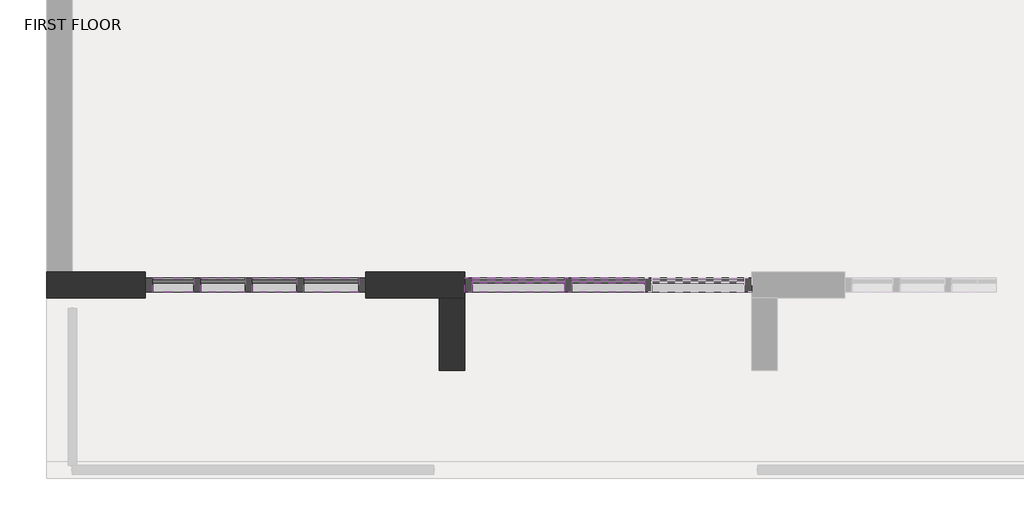
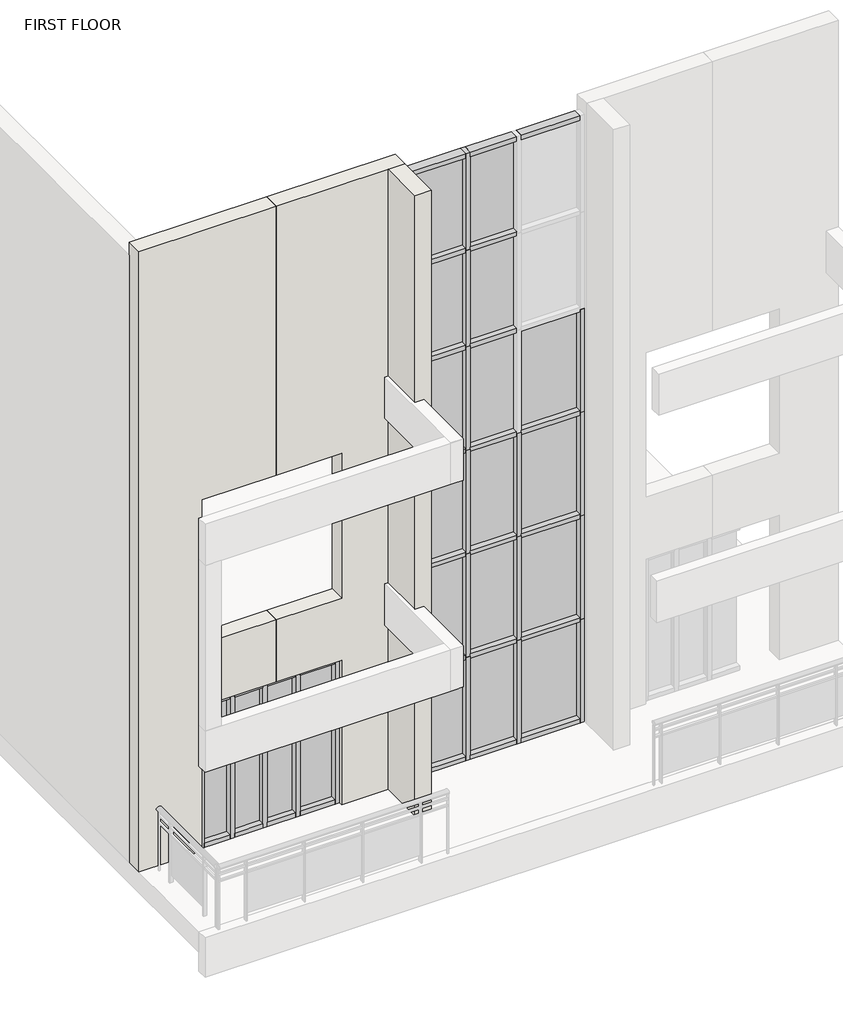
# One storey, part 1 of 2: 64 members, 24 plates, 3 walls.
"""IFC4 building model written with IfcOpenShell, lengths in millimetres."""

from ifc_helpers import new_model, si_unit, frame, origin, place, context, project, spatial, polyline, outline, extrude, faceted_brep, transform, mapped, element, save
from components import member_3374d9b6, member_c17f1be2, member_5215b92c, member_82905deb, member_ad567e07, member_e53b78c9, member_4491d118, member_0514ece2, member_5493b72c, member_7cbddb58, member_843225dc, member_7096a90e, member_499db0bc, system_panel_glazed_d26374ee, system_panel_glazed_59bf60dd, system_panel_glazed_016e6134, system_panel_glazed_b44f8fb5, system_panel_glazed_3f785c8f, system_panel_glazed_bf013b5c, system_panel_glazed_d91b2d6b, system_panel_glazed_ad4bb790, system_panel_glazed_935821d8, system_panel_glazed_f3f5655f, system_panel_glazed_1490133a

model = new_model("IFC4")

# Units and contexts
model_context = context("Model", 3, world=origin())
ifc_project = project(units=[si_unit("LENGTHUNIT", "METRE", prefix="MILLI")], contexts=[model_context])

# Site, building, storey
site = spatial("IfcSite", under=ifc_project)
building = spatial("IfcBuilding", under=site)
storey = spatial("IfcBuildingStorey", under=building, Name="FIRST FLOOR", Elevation=3048.0)

# Members
placement = place(None, origin())
member_shape = member_3374d9b6(model_context)
element("IfcMember", 1, ObjectType="Rectangular Mullion : 2.5\" x 5\" rectangular", at=placement, inside=storey, context=model_context, shape_type="MappedRepresentation", body=[
    mapped(member_shape, transform((-3493.058803, -508.3464931, 3048.0), x_axis=(1.0, 0.0, 0.0), y_axis=(0.0, -1.0, 0.0), z_axis=(0.0, 0.0, -1.0))),
])
element("IfcMember", 2, ObjectType="Rectangular Mullion : 2.5\" x 5\" rectangular", at=placement, inside=storey, context=model_context, shape_type="MappedRepresentation", body=[
    mapped(member_shape, transform((-3493.058803, -508.3464931, 3048.0), x_axis=(1.0, 0.0, 0.0), y_axis=(0.0, -1.0, 0.0), z_axis=(0.0, 0.0, -1.0))),
])
element("IfcMember", 3, ObjectType="Rectangular Mullion : 2.5\" x 5\" rectangular", at=placement, inside=storey, context=model_context, shape_type="MappedRepresentation", body=[
    mapped(member_shape, transform((-5445.7230786, -508.3464931, 5181.6), x_axis=(-1.0, 0.0, 0.0), y_axis=(0.0, -1.0, 0.0), z_axis=(0.0, 0.0, 1.0))),
])
element("IfcMember", 4, ObjectType="Rectangular Mullion : 2.5\" x 5\" rectangular", at=placement, inside=storey, context=model_context, shape_type="MappedRepresentation", body=[
    mapped(member_shape, transform((-5445.7230786, -508.3464931, 5181.6), x_axis=(-1.0, 0.0, 0.0), y_axis=(0.0, -1.0, 0.0), z_axis=(0.0, 0.0, 1.0))),
])
member_2_shape = member_c17f1be2(model_context)
element("IfcMember", 5, ObjectType="Rectangular Mullion : 2.5\" x 5\" rectangular", at=placement, inside=storey, context=model_context, shape_type="MappedRepresentation", body=[
    mapped(member_2_shape, transform((-2553.258803, -508.3464931, 3048.0), x_axis=(0.0, 0.0, -1.0), y_axis=(0.0, -1.0, 0.0), z_axis=(-1.0, 0.0, 0.0))),
])
element("IfcMember", 6, ObjectType="Rectangular Mullion : 2.5\" x 5\" rectangular", at=placement, inside=storey, context=model_context, shape_type="MappedRepresentation", body=[
    mapped(member_2_shape, transform((-959.408803, -508.3464931, 3048.0), x_axis=(0.0, 0.0, -1.0), y_axis=(0.0, -1.0, 0.0), z_axis=(-1.0, 0.0, 0.0))),
])
element("IfcMember", 7, ObjectType="Rectangular Mullion : 2.5\" x 5\" rectangular", at=placement, inside=storey, context=model_context, shape_type="MappedRepresentation", body=[
    mapped(member_2_shape, transform((-140.258803, -508.3464931, 12000.3983116), x_axis=(0.0, 0.0, 1.0), y_axis=(0.0, -1.0, 0.0), z_axis=(1.0, 0.0, 0.0))),
])
element("IfcMember", 8, ObjectType="Rectangular Mullion : 2.5\" x 5\" rectangular", at=placement, inside=storey, context=model_context, shape_type="MappedRepresentation", body=[
    mapped(member_2_shape, transform((-1734.108803, -508.3464931, 12000.3983116), x_axis=(0.0, 0.0, 1.0), y_axis=(0.0, -1.0, 0.0), z_axis=(1.0, 0.0, 0.0))),
])
member_3_shape = member_5215b92c(model_context)
element("IfcMember", 9, ObjectType="Rectangular Mullion : 2.5\" x 5\" rectangular", at=placement, inside=storey, context=model_context, shape_type="MappedRepresentation", body=[
    mapped(member_3_shape, transform((-1670.608803, -508.3464931, 3048.0), x_axis=(0.0, 0.0, -1.0), y_axis=(0.0, -1.0, 0.0), z_axis=(-1.0, 0.0, 0.0))),
])
element("IfcMember", 10, ObjectType="Rectangular Mullion : 2.5\" x 5\" rectangular", at=placement, inside=storey, context=model_context, shape_type="MappedRepresentation", body=[
    mapped(member_3_shape, transform((-1022.908803, -508.3464931, 12000.3983116), x_axis=(0.0, 0.0, 1.0), y_axis=(0.0, -1.0, 0.0), z_axis=(1.0, 0.0, 0.0))),
])
member_4_shape = member_82905deb(model_context)
element("IfcMember", 11, ObjectType="Rectangular Mullion : 2.5\" x 5\" rectangular", at=placement, inside=storey, context=model_context, shape_type="MappedRepresentation", body=[
    mapped(member_4_shape, transform((-1702.358803, -508.3464931, 3048.0), x_axis=(1.0, 0.0, 0.0), y_axis=(0.0, -1.0, 0.0), z_axis=(0.0, 0.0, -1.0))),
])
element("IfcMember", 12, ObjectType="Rectangular Mullion : 2.5\" x 5\" rectangular", at=placement, inside=storey, context=model_context, shape_type="MappedRepresentation", body=[
    mapped(member_4_shape, transform((-991.158803, -508.3464931, 3048.0), x_axis=(1.0, 0.0, 0.0), y_axis=(0.0, -1.0, 0.0), z_axis=(0.0, 0.0, -1.0))),
])
member_5_shape = member_ad567e07(model_context)
element("IfcMember", 13, ObjectType="Rectangular Mullion : 2.5\" x 5\" rectangular", at=placement, inside=storey, context=model_context, shape_type="MappedRepresentation", body=[
    mapped(member_5_shape, transform((-1734.108803, -508.3464931, 4572.0), x_axis=(0.0, 0.0, 1.0), y_axis=(0.0, -1.0, 0.0), z_axis=(1.0, 0.0, 0.0))),
])
element("IfcMember", 14, ObjectType="Rectangular Mullion : 2.5\" x 5\" rectangular", at=placement, inside=storey, context=model_context, shape_type="MappedRepresentation", body=[
    mapped(member_5_shape, transform((-140.258803, -508.3464931, 4572.0), x_axis=(0.0, 0.0, 1.0), y_axis=(0.0, -1.0, 0.0), z_axis=(1.0, 0.0, 0.0))),
])
element("IfcMember", 15, ObjectType="Rectangular Mullion : 2.5\" x 5\" rectangular", at=placement, inside=storey, context=model_context, shape_type="MappedRepresentation", body=[
    mapped(member_5_shape, transform((-1734.108803, -508.3464931, 6096.0), x_axis=(0.0, 0.0, 1.0), y_axis=(0.0, -1.0, 0.0), z_axis=(1.0, 0.0, 0.0))),
])
element("IfcMember", 16, ObjectType="Rectangular Mullion : 2.5\" x 5\" rectangular", at=placement, inside=storey, context=model_context, shape_type="MappedRepresentation", body=[
    mapped(member_5_shape, transform((-140.258803, -508.3464931, 6096.0), x_axis=(0.0, 0.0, 1.0), y_axis=(0.0, -1.0, 0.0), z_axis=(1.0, 0.0, 0.0))),
])
element("IfcMember", 17, ObjectType="Rectangular Mullion : 2.5\" x 5\" rectangular", at=placement, inside=storey, context=model_context, shape_type="MappedRepresentation", body=[
    mapped(member_5_shape, transform((-1734.108803, -508.3464931, 7620.0), x_axis=(0.0, 0.0, 1.0), y_axis=(0.0, -1.0, 0.0), z_axis=(1.0, 0.0, 0.0))),
])
element("IfcMember", 18, ObjectType="Rectangular Mullion : 2.5\" x 5\" rectangular", at=placement, inside=storey, context=model_context, shape_type="MappedRepresentation", body=[
    mapped(member_5_shape, transform((-140.258803, -508.3464931, 7620.0), x_axis=(0.0, 0.0, 1.0), y_axis=(0.0, -1.0, 0.0), z_axis=(1.0, 0.0, 0.0))),
])
element("IfcMember", 19, ObjectType="Rectangular Mullion : 2.5\" x 5\" rectangular", at=placement, inside=storey, context=model_context, shape_type="MappedRepresentation", body=[
    mapped(member_5_shape, transform((-1734.108803, -508.3464931, 9144.0), x_axis=(0.0, 0.0, 1.0), y_axis=(0.0, -1.0, 0.0), z_axis=(1.0, 0.0, 0.0))),
])
element("IfcMember", 20, ObjectType="Rectangular Mullion : 2.5\" x 5\" rectangular", at=placement, inside=storey, context=model_context, shape_type="MappedRepresentation", body=[
    mapped(member_5_shape, transform((-1734.108803, -508.3464931, 10572.1991558), x_axis=(0.0, 0.0, 1.0), y_axis=(0.0, -1.0, 0.0), z_axis=(1.0, 0.0, 0.0))),
])
member_6_shape = member_e53b78c9(model_context)
element("IfcMember", 21, ObjectType="Rectangular Mullion : 2.5\" x 5\" rectangular", at=placement, inside=storey, context=model_context, shape_type="MappedRepresentation", body=[
    mapped(member_6_shape, transform((-1022.908803, -508.3464931, 4572.0), x_axis=(0.0, 0.0, 1.0), y_axis=(0.0, -1.0, 0.0), z_axis=(1.0, 0.0, 0.0))),
])
element("IfcMember", 22, ObjectType="Rectangular Mullion : 2.5\" x 5\" rectangular", at=placement, inside=storey, context=model_context, shape_type="MappedRepresentation", body=[
    mapped(member_6_shape, transform((-1022.908803, -508.3464931, 6096.0), x_axis=(0.0, 0.0, 1.0), y_axis=(0.0, -1.0, 0.0), z_axis=(1.0, 0.0, 0.0))),
])
element("IfcMember", 23, ObjectType="Rectangular Mullion : 2.5\" x 5\" rectangular", at=placement, inside=storey, context=model_context, shape_type="MappedRepresentation", body=[
    mapped(member_6_shape, transform((-1022.908803, -508.3464931, 7620.0), x_axis=(0.0, 0.0, 1.0), y_axis=(0.0, -1.0, 0.0), z_axis=(1.0, 0.0, 0.0))),
])
element("IfcMember", 24, ObjectType="Rectangular Mullion : 2.5\" x 5\" rectangular", at=placement, inside=storey, context=model_context, shape_type="MappedRepresentation", body=[
    mapped(member_6_shape, transform((-1022.908803, -508.3464931, 9144.0), x_axis=(0.0, 0.0, 1.0), y_axis=(0.0, -1.0, 0.0), z_axis=(1.0, 0.0, 0.0))),
])
element("IfcMember", 25, ObjectType="Rectangular Mullion : 2.5\" x 5\" rectangular", at=placement, inside=storey, context=model_context, shape_type="MappedRepresentation", body=[
    mapped(member_6_shape, transform((-1022.908803, -508.3464931, 10572.1991558), x_axis=(0.0, 0.0, 1.0), y_axis=(0.0, -1.0, 0.0), z_axis=(1.0, 0.0, 0.0))),
])
member_7_shape = member_4491d118(model_context)
element("IfcMember", 26, ObjectType="Rectangular Mullion : 2.5\" x 5\" rectangular", at=placement, inside=storey, context=model_context, shape_type="MappedRepresentation", body=[
    mapped(member_7_shape, transform((-76.758803, -508.3464931, 3048.0), x_axis=(1.0, 0.0, 0.0), y_axis=(0.0, -1.0, 0.0), z_axis=(0.0, 0.0, -1.0))),
])
element("IfcMember", 27, ObjectType="Rectangular Mullion : 2.5\" x 5\" rectangular", at=placement, inside=storey, context=model_context, shape_type="MappedRepresentation", body=[
    mapped(member_7_shape, transform((-2616.758803, -508.3464931, 4572.0), x_axis=(-1.0, 0.0, 0.0), y_axis=(0.0, -1.0, 0.0), z_axis=(0.0, 0.0, 1.0))),
])
element("IfcMember", 28, ObjectType="Rectangular Mullion : 2.5\" x 5\" rectangular", at=placement, inside=storey, context=model_context, shape_type="MappedRepresentation", body=[
    mapped(member_4_shape, transform((-1702.358803, -508.3464931, 4572.0), x_axis=(1.0, 0.0, 0.0), y_axis=(0.0, -1.0, 0.0), z_axis=(0.0, 0.0, -1.0))),
])
element("IfcMember", 29, ObjectType="Rectangular Mullion : 2.5\" x 5\" rectangular", at=placement, inside=storey, context=model_context, shape_type="MappedRepresentation", body=[
    mapped(member_4_shape, transform((-991.158803, -508.3464931, 4572.0), x_axis=(1.0, 0.0, 0.0), y_axis=(0.0, -1.0, 0.0), z_axis=(0.0, 0.0, -1.0))),
])
element("IfcMember", 30, ObjectType="Rectangular Mullion : 2.5\" x 5\" rectangular", at=placement, inside=storey, context=model_context, shape_type="MappedRepresentation", body=[
    mapped(member_4_shape, transform((-1702.358803, -508.3464931, 6096.0), x_axis=(1.0, 0.0, 0.0), y_axis=(0.0, -1.0, 0.0), z_axis=(0.0, 0.0, -1.0))),
])
element("IfcMember", 31, ObjectType="Rectangular Mullion : 2.5\" x 5\" rectangular", at=placement, inside=storey, context=model_context, shape_type="MappedRepresentation", body=[
    mapped(member_4_shape, transform((-991.158803, -508.3464931, 6096.0), x_axis=(1.0, 0.0, 0.0), y_axis=(0.0, -1.0, 0.0), z_axis=(0.0, 0.0, -1.0))),
])
element("IfcMember", 32, ObjectType="Rectangular Mullion : 2.5\" x 5\" rectangular", at=placement, inside=storey, context=model_context, shape_type="MappedRepresentation", body=[
    mapped(member_4_shape, transform((-1702.358803, -508.3464931, 7620.0), x_axis=(1.0, 0.0, 0.0), y_axis=(0.0, -1.0, 0.0), z_axis=(0.0, 0.0, -1.0))),
])
element("IfcMember", 33, ObjectType="Rectangular Mullion : 2.5\" x 5\" rectangular", at=placement, inside=storey, context=model_context, shape_type="MappedRepresentation", body=[
    mapped(member_7_shape, transform((-76.758803, -508.3464931, 4572.0), x_axis=(1.0, 0.0, 0.0), y_axis=(0.0, -1.0, 0.0), z_axis=(0.0, 0.0, -1.0))),
])
element("IfcMember", 34, ObjectType="Rectangular Mullion : 2.5\" x 5\" rectangular", at=placement, inside=storey, context=model_context, shape_type="MappedRepresentation", body=[
    mapped(member_7_shape, transform((-76.758803, -508.3464931, 6096.0), x_axis=(1.0, 0.0, 0.0), y_axis=(0.0, -1.0, 0.0), z_axis=(0.0, 0.0, -1.0))),
])
element("IfcMember", 35, ObjectType="Rectangular Mullion : 2.5\" x 5\" rectangular", at=placement, inside=storey, context=model_context, shape_type="MappedRepresentation", body=[
    mapped(member_7_shape, transform((-76.758803, -508.3464931, 7620.0), x_axis=(1.0, 0.0, 0.0), y_axis=(0.0, -1.0, 0.0), z_axis=(0.0, 0.0, -1.0))),
])
element("IfcMember", 36, ObjectType="Rectangular Mullion : 2.5\" x 5\" rectangular", at=placement, inside=storey, context=model_context, shape_type="MappedRepresentation", body=[
    mapped(member_7_shape, transform((-2616.758803, -508.3464931, 6096.0), x_axis=(-1.0, 0.0, 0.0), y_axis=(0.0, -1.0, 0.0), z_axis=(0.0, 0.0, 1.0))),
])
element("IfcMember", 37, ObjectType="Rectangular Mullion : 2.5\" x 5\" rectangular", at=placement, inside=storey, context=model_context, shape_type="MappedRepresentation", body=[
    mapped(member_7_shape, transform((-2616.758803, -508.3464931, 7620.0), x_axis=(-1.0, 0.0, 0.0), y_axis=(0.0, -1.0, 0.0), z_axis=(0.0, 0.0, 1.0))),
])
element("IfcMember", 38, ObjectType="Rectangular Mullion : 2.5\" x 5\" rectangular", at=placement, inside=storey, context=model_context, shape_type="MappedRepresentation", body=[
    mapped(member_7_shape, transform((-2616.758803, -508.3464931, 9144.0), x_axis=(-1.0, 0.0, 0.0), y_axis=(0.0, -1.0, 0.0), z_axis=(0.0, 0.0, 1.0))),
])
member_8_shape = member_0514ece2(model_context)
element("IfcMember", 39, ObjectType="Rectangular Mullion : 2.5\" x 5\" rectangular", at=placement, inside=storey, context=model_context, shape_type="MappedRepresentation", body=[
    mapped(member_8_shape, transform((-1702.358803, -508.3464931, 9144.0), x_axis=(1.0, 0.0, 0.0), y_axis=(0.0, -1.0, 0.0), z_axis=(0.0, 0.0, -1.0))),
])
element("IfcMember", 40, ObjectType="Rectangular Mullion : 2.5\" x 5\" rectangular", at=placement, inside=storey, context=model_context, shape_type="MappedRepresentation", body=[
    mapped(member_8_shape, transform((-1702.358803, -508.3464931, 10572.1991558), x_axis=(1.0, 0.0, 0.0), y_axis=(0.0, -1.0, 0.0), z_axis=(0.0, 0.0, -1.0))),
])
member_9_shape = member_5493b72c(model_context)
element("IfcMember", 41, ObjectType="Rectangular Mullion : 2.5\" x 5\" rectangular", at=placement, inside=storey, context=model_context, shape_type="MappedRepresentation", body=[
    mapped(member_9_shape, transform((-2616.758803, -508.3464931, 12000.3983116), x_axis=(-1.0, 0.0, 0.0), y_axis=(0.0, -1.0, 0.0), z_axis=(0.0, 0.0, 1.0))),
])
element("IfcMember", 42, ObjectType="Rectangular Mullion : 2.5\" x 5\" rectangular", at=placement, inside=storey, context=model_context, shape_type="MappedRepresentation", body=[
    mapped(member_9_shape, transform((-2616.758803, -508.3464931, 10572.1991558), x_axis=(-1.0, 0.0, 0.0), y_axis=(0.0, -1.0, 0.0), z_axis=(0.0, 0.0, 1.0))),
])
member_10_shape = member_7cbddb58(model_context)
element("IfcMember", 43, ObjectType="Rectangular Mullion : 2.5\" x 5\" rectangular", at=placement, inside=storey, context=model_context, shape_type="MappedRepresentation", body=[
    mapped(member_10_shape, transform((-4988.5230786, -508.3464931, 3048.0), x_axis=(1.0, 0.0, 0.0), y_axis=(0.0, -1.0, 0.0), z_axis=(0.0, 0.0, -1.0))),
])
element("IfcMember", 44, ObjectType="Rectangular Mullion : 2.5\" x 5\" rectangular", at=placement, inside=storey, context=model_context, shape_type="MappedRepresentation", body=[
    mapped(member_10_shape, transform((-4531.3230786, -508.3464931, 3048.0), x_axis=(1.0, 0.0, 0.0), y_axis=(0.0, -1.0, 0.0), z_axis=(0.0, 0.0, -1.0))),
])
element("IfcMember", 45, ObjectType="Rectangular Mullion : 2.5\" x 5\" rectangular", at=placement, inside=storey, context=model_context, shape_type="MappedRepresentation", body=[
    mapped(member_10_shape, transform((-4074.1230786, -508.3464931, 3048.0), x_axis=(1.0, 0.0, 0.0), y_axis=(0.0, -1.0, 0.0), z_axis=(0.0, 0.0, -1.0))),
])
element("IfcMember", 46, ObjectType="Rectangular Mullion : 2.5\" x 5\" rectangular", at=placement, inside=storey, context=model_context, shape_type="MappedRepresentation", body=[
    mapped(member_10_shape, transform((-4988.5230786, -508.3464931, 3048.0), x_axis=(1.0, 0.0, 0.0), y_axis=(0.0, -1.0, 0.0), z_axis=(0.0, 0.0, -1.0))),
])
element("IfcMember", 47, ObjectType="Rectangular Mullion : 2.5\" x 5\" rectangular", at=placement, inside=storey, context=model_context, shape_type="MappedRepresentation", body=[
    mapped(member_10_shape, transform((-4531.3230786, -508.3464931, 3048.0), x_axis=(1.0, 0.0, 0.0), y_axis=(0.0, -1.0, 0.0), z_axis=(0.0, 0.0, -1.0))),
])
element("IfcMember", 48, ObjectType="Rectangular Mullion : 2.5\" x 5\" rectangular", at=placement, inside=storey, context=model_context, shape_type="MappedRepresentation", body=[
    mapped(member_10_shape, transform((-4074.1230786, -508.3464931, 3048.0), x_axis=(1.0, 0.0, 0.0), y_axis=(0.0, -1.0, 0.0), z_axis=(0.0, 0.0, -1.0))),
])
member_11_shape = member_843225dc(model_context)
element("IfcMember", 49, ObjectType="Rectangular Mullion : 2.5\" x 5\" rectangular", at=placement, inside=storey, context=model_context, shape_type="MappedRepresentation", body=[
    mapped(member_11_shape, transform((-5382.2230786, -508.3464931, 3048.0), x_axis=(0.0, 0.0, -1.0), y_axis=(0.0, -1.0, 0.0), z_axis=(-1.0, 0.0, 0.0))),
])
element("IfcMember", 50, ObjectType="Rectangular Mullion : 2.5\" x 5\" rectangular", at=placement, inside=storey, context=model_context, shape_type="MappedRepresentation", body=[
    mapped(member_11_shape, transform((-5382.2230786, -508.3464931, 3048.0), x_axis=(0.0, 0.0, -1.0), y_axis=(0.0, -1.0, 0.0), z_axis=(-1.0, 0.0, 0.0))),
])
element("IfcMember", 51, ObjectType="Rectangular Mullion : 2.5\" x 5\" rectangular", at=placement, inside=storey, context=model_context, shape_type="MappedRepresentation", body=[
    mapped(member_11_shape, transform((-5020.2730786, -508.3464931, 5181.6), x_axis=(0.0, 0.0, 1.0), y_axis=(0.0, -1.0, 0.0), z_axis=(1.0, 0.0, 0.0))),
])
element("IfcMember", 52, ObjectType="Rectangular Mullion : 2.5\" x 5\" rectangular", at=placement, inside=storey, context=model_context, shape_type="MappedRepresentation", body=[
    mapped(member_11_shape, transform((-5020.2730786, -508.3464931, 5181.6), x_axis=(0.0, 0.0, 1.0), y_axis=(0.0, -1.0, 0.0), z_axis=(1.0, 0.0, 0.0))),
])
member_12_shape = member_7096a90e(model_context)
element("IfcMember", 53, ObjectType="Rectangular Mullion : 2.5\" x 5\" rectangular", at=placement, inside=storey, context=model_context, shape_type="MappedRepresentation", body=[
    mapped(member_12_shape, transform((-4956.7730786, -508.3464931, 3048.0), x_axis=(0.0, 0.0, -1.0), y_axis=(0.0, -1.0, 0.0), z_axis=(-1.0, 0.0, 0.0))),
])
element("IfcMember", 54, ObjectType="Rectangular Mullion : 2.5\" x 5\" rectangular", at=placement, inside=storey, context=model_context, shape_type="MappedRepresentation", body=[
    mapped(member_12_shape, transform((-4499.5730786, -508.3464931, 3048.0), x_axis=(0.0, 0.0, -1.0), y_axis=(0.0, -1.0, 0.0), z_axis=(-1.0, 0.0, 0.0))),
])
element("IfcMember", 55, ObjectType="Rectangular Mullion : 2.5\" x 5\" rectangular", at=placement, inside=storey, context=model_context, shape_type="MappedRepresentation", body=[
    mapped(member_12_shape, transform((-4956.7730786, -508.3464931, 3048.0), x_axis=(0.0, 0.0, -1.0), y_axis=(0.0, -1.0, 0.0), z_axis=(-1.0, 0.0, 0.0))),
])
element("IfcMember", 56, ObjectType="Rectangular Mullion : 2.5\" x 5\" rectangular", at=placement, inside=storey, context=model_context, shape_type="MappedRepresentation", body=[
    mapped(member_12_shape, transform((-4499.5730786, -508.3464931, 3048.0), x_axis=(0.0, 0.0, -1.0), y_axis=(0.0, -1.0, 0.0), z_axis=(-1.0, 0.0, 0.0))),
])
element("IfcMember", 57, ObjectType="Rectangular Mullion : 2.5\" x 5\" rectangular", at=placement, inside=storey, context=model_context, shape_type="MappedRepresentation", body=[
    mapped(member_12_shape, transform((-4563.0730786, -508.3464931, 5181.6), x_axis=(0.0, 0.0, 1.0), y_axis=(0.0, -1.0, 0.0), z_axis=(1.0, 0.0, 0.0))),
])
element("IfcMember", 58, ObjectType="Rectangular Mullion : 2.5\" x 5\" rectangular", at=placement, inside=storey, context=model_context, shape_type="MappedRepresentation", body=[
    mapped(member_12_shape, transform((-4105.8730786, -508.3464931, 5181.6), x_axis=(0.0, 0.0, 1.0), y_axis=(0.0, -1.0, 0.0), z_axis=(1.0, 0.0, 0.0))),
])
element("IfcMember", 59, ObjectType="Rectangular Mullion : 2.5\" x 5\" rectangular", at=placement, inside=storey, context=model_context, shape_type="MappedRepresentation", body=[
    mapped(member_12_shape, transform((-4563.0730786, -508.3464931, 5181.6), x_axis=(0.0, 0.0, 1.0), y_axis=(0.0, -1.0, 0.0), z_axis=(1.0, 0.0, 0.0))),
])
element("IfcMember", 60, ObjectType="Rectangular Mullion : 2.5\" x 5\" rectangular", at=placement, inside=storey, context=model_context, shape_type="MappedRepresentation", body=[
    mapped(member_12_shape, transform((-4105.8730786, -508.3464931, 5181.6), x_axis=(0.0, 0.0, 1.0), y_axis=(0.0, -1.0, 0.0), z_axis=(1.0, 0.0, 0.0))),
])
member_13_shape = member_499db0bc(model_context)
element("IfcMember", 61, ObjectType="Rectangular Mullion : 2.5\" x 5\" rectangular", at=placement, inside=storey, context=model_context, shape_type="MappedRepresentation", body=[
    mapped(member_13_shape, transform((-3556.558803, -508.3464931, 5181.6), x_axis=(0.0, 0.0, 1.0), y_axis=(0.0, -1.0, 0.0), z_axis=(1.0, 0.0, 0.0))),
])
element("IfcMember", 62, ObjectType="Rectangular Mullion : 2.5\" x 5\" rectangular", at=placement, inside=storey, context=model_context, shape_type="MappedRepresentation", body=[
    mapped(member_13_shape, transform((-3556.558803, -508.3464931, 5181.6), x_axis=(0.0, 0.0, 1.0), y_axis=(0.0, -1.0, 0.0), z_axis=(1.0, 0.0, 0.0))),
])
element("IfcMember", 63, ObjectType="Rectangular Mullion : 2.5\" x 5\" rectangular", at=placement, inside=storey, context=model_context, shape_type="MappedRepresentation", body=[
    mapped(member_13_shape, transform((-4042.3730786, -508.3464931, 3048.0), x_axis=(0.0, 0.0, -1.0), y_axis=(0.0, -1.0, 0.0), z_axis=(-1.0, 0.0, 0.0))),
])
element("IfcMember", 64, ObjectType="Rectangular Mullion : 2.5\" x 5\" rectangular", at=placement, inside=storey, context=model_context, shape_type="MappedRepresentation", body=[
    mapped(member_13_shape, transform((-4042.3730786, -508.3464931, 3048.0), x_axis=(0.0, 0.0, -1.0), y_axis=(0.0, -1.0, 0.0), z_axis=(-1.0, 0.0, 0.0))),
])

# Plates
system_panel_glazed_shape = system_panel_glazed_d26374ee(model_context)
element("IfcPlate", 65, ObjectType="System Panel : Glazed", at=placement, inside=storey, context=model_context, shape_type="MappedRepresentation", body=[
    mapped(system_panel_glazed_shape, transform((-2143.683803, -508.3464931, 3111.5), x_axis=(1.0, 0.0, 0.0), y_axis=(0.0, 1.0, 0.0), z_axis=(0.0, 0.0, 1.0))),
])
element("IfcPlate", 66, ObjectType="System Panel : Glazed", at=placement, inside=storey, context=model_context, shape_type="MappedRepresentation", body=[
    mapped(system_panel_glazed_shape, transform((-549.833803, -508.3464931, 3111.5), x_axis=(1.0, 0.0, 0.0), y_axis=(0.0, 1.0, 0.0), z_axis=(0.0, 0.0, 1.0))),
])
system_panel_glazed_2_shape = system_panel_glazed_59bf60dd(model_context)
element("IfcPlate", 67, ObjectType="System Panel : Glazed", at=placement, inside=storey, context=model_context, shape_type="MappedRepresentation", body=[
    mapped(system_panel_glazed_2_shape, transform((-1346.758803, -508.3464931, 3111.5), x_axis=(1.0, 0.0, 0.0), y_axis=(0.0, 1.0, 0.0), z_axis=(0.0, 0.0, 1.0))),
])
system_panel_glazed_3_shape = system_panel_glazed_016e6134(model_context)
element("IfcPlate", 68, ObjectType="System Panel : Glazed", at=placement, inside=storey, context=model_context, shape_type="MappedRepresentation", body=[
    mapped(system_panel_glazed_3_shape, transform((-2143.683803, -508.3464931, 4603.75), x_axis=(1.0, 0.0, 0.0), y_axis=(0.0, 1.0, 0.0), z_axis=(0.0, 0.0, 1.0))),
])
element("IfcPlate", 69, ObjectType="System Panel : Glazed", at=placement, inside=storey, context=model_context, shape_type="MappedRepresentation", body=[
    mapped(system_panel_glazed_3_shape, transform((-549.833803, -508.3464931, 4603.75), x_axis=(1.0, 0.0, 0.0), y_axis=(0.0, 1.0, 0.0), z_axis=(0.0, 0.0, 1.0))),
])
element("IfcPlate", 70, ObjectType="System Panel : Glazed", at=placement, inside=storey, context=model_context, shape_type="MappedRepresentation", body=[
    mapped(system_panel_glazed_3_shape, transform((-2143.683803, -508.3464931, 6127.75), x_axis=(1.0, 0.0, 0.0), y_axis=(0.0, 1.0, 0.0), z_axis=(0.0, 0.0, 1.0))),
])
element("IfcPlate", 71, ObjectType="System Panel : Glazed", at=placement, inside=storey, context=model_context, shape_type="MappedRepresentation", body=[
    mapped(system_panel_glazed_3_shape, transform((-549.833803, -508.3464931, 6127.75), x_axis=(1.0, 0.0, 0.0), y_axis=(0.0, 1.0, 0.0), z_axis=(0.0, 0.0, 1.0))),
])
element("IfcPlate", 72, ObjectType="System Panel : Glazed", at=placement, inside=storey, context=model_context, shape_type="MappedRepresentation", body=[
    mapped(system_panel_glazed_3_shape, transform((-2143.683803, -508.3464931, 7651.75), x_axis=(1.0, 0.0, 0.0), y_axis=(0.0, 1.0, 0.0), z_axis=(0.0, 0.0, 1.0))),
])
element("IfcPlate", 73, ObjectType="System Panel : Glazed", at=placement, inside=storey, context=model_context, shape_type="MappedRepresentation", body=[
    mapped(system_panel_glazed_3_shape, transform((-549.833803, -508.3464931, 7651.75), x_axis=(1.0, 0.0, 0.0), y_axis=(0.0, 1.0, 0.0), z_axis=(0.0, 0.0, 1.0))),
])
system_panel_glazed_4_shape = system_panel_glazed_b44f8fb5(model_context)
element("IfcPlate", 74, ObjectType="System Panel : Glazed", at=placement, inside=storey, context=model_context, shape_type="MappedRepresentation", body=[
    mapped(system_panel_glazed_4_shape, transform((-1346.758803, -508.3464931, 4603.75), x_axis=(1.0, 0.0, 0.0), y_axis=(0.0, 1.0, 0.0), z_axis=(0.0, 0.0, 1.0))),
])
element("IfcPlate", 75, ObjectType="System Panel : Glazed", at=placement, inside=storey, context=model_context, shape_type="MappedRepresentation", body=[
    mapped(system_panel_glazed_4_shape, transform((-1346.758803, -508.3464931, 6127.75), x_axis=(1.0, 0.0, 0.0), y_axis=(0.0, 1.0, 0.0), z_axis=(0.0, 0.0, 1.0))),
])
element("IfcPlate", 76, ObjectType="System Panel : Glazed", at=placement, inside=storey, context=model_context, shape_type="MappedRepresentation", body=[
    mapped(system_panel_glazed_4_shape, transform((-1346.758803, -508.3464931, 7651.75), x_axis=(1.0, 0.0, 0.0), y_axis=(0.0, 1.0, 0.0), z_axis=(0.0, 0.0, 1.0))),
])
system_panel_glazed_5_shape = system_panel_glazed_3f785c8f(model_context)
element("IfcPlate", 77, ObjectType="System Panel : Glazed", at=placement, inside=storey, context=model_context, shape_type="MappedRepresentation", body=[
    mapped(system_panel_glazed_5_shape, transform((-2143.683803, -508.3464931, 9175.75), x_axis=(1.0, 0.0, 0.0), y_axis=(0.0, 1.0, 0.0), z_axis=(0.0, 0.0, 1.0))),
])
system_panel_glazed_6_shape = system_panel_glazed_bf013b5c(model_context)
element("IfcPlate", 78, ObjectType="System Panel : Glazed", at=placement, inside=storey, context=model_context, shape_type="MappedRepresentation", body=[
    mapped(system_panel_glazed_6_shape, transform((-1346.758803, -508.3464931, 9175.75), x_axis=(1.0, 0.0, 0.0), y_axis=(0.0, 1.0, 0.0), z_axis=(0.0, 0.0, 1.0))),
])
system_panel_glazed_7_shape = system_panel_glazed_d91b2d6b(model_context)
element("IfcPlate", 79, ObjectType="System Panel : Glazed", at=placement, inside=storey, context=model_context, shape_type="MappedRepresentation", body=[
    mapped(system_panel_glazed_7_shape, transform((-2143.683803, -508.3464931, 10603.9491558), x_axis=(1.0, 0.0, 0.0), y_axis=(0.0, 1.0, 0.0), z_axis=(0.0, 0.0, 1.0))),
])
system_panel_glazed_8_shape = system_panel_glazed_ad4bb790(model_context)
element("IfcPlate", 80, ObjectType="System Panel : Glazed", at=placement, inside=storey, context=model_context, shape_type="MappedRepresentation", body=[
    mapped(system_panel_glazed_8_shape, transform((-1346.758803, -508.3464931, 10603.9491558), x_axis=(1.0, 0.0, 0.0), y_axis=(0.0, 1.0, 0.0), z_axis=(0.0, 0.0, 1.0))),
])
system_panel_glazed_9_shape = system_panel_glazed_935821d8(model_context)
element("IfcPlate", 81, ObjectType="System Panel : Glazed", at=placement, inside=storey, context=model_context, shape_type="MappedRepresentation", body=[
    mapped(system_panel_glazed_9_shape, transform((-5201.2480786, -508.3464931, 3111.5), x_axis=(1.0, 0.0, 0.0), y_axis=(0.0, 1.0, 0.0), z_axis=(0.0, 0.0, 1.0))),
])
element("IfcPlate", 82, ObjectType="System Panel : Glazed", at=placement, inside=storey, context=model_context, shape_type="MappedRepresentation", body=[
    mapped(system_panel_glazed_9_shape, transform((-5201.2480786, -508.3464931, 3111.5), x_axis=(1.0, 0.0, 0.0), y_axis=(0.0, 1.0, 0.0), z_axis=(0.0, 0.0, 1.0))),
])
system_panel_glazed_10_shape = system_panel_glazed_f3f5655f(model_context)
element("IfcPlate", 83, ObjectType="System Panel : Glazed", at=placement, inside=storey, context=model_context, shape_type="MappedRepresentation", body=[
    mapped(system_panel_glazed_10_shape, transform((-4759.9230786, -508.3464931, 3111.5), x_axis=(1.0, 0.0, 0.0), y_axis=(0.0, 1.0, 0.0), z_axis=(0.0, 0.0, 1.0))),
])
element("IfcPlate", 84, ObjectType="System Panel : Glazed", at=placement, inside=storey, context=model_context, shape_type="MappedRepresentation", body=[
    mapped(system_panel_glazed_10_shape, transform((-4302.7230786, -508.3464931, 3111.5), x_axis=(1.0, 0.0, 0.0), y_axis=(0.0, 1.0, 0.0), z_axis=(0.0, 0.0, 1.0))),
])
element("IfcPlate", 85, ObjectType="System Panel : Glazed", at=placement, inside=storey, context=model_context, shape_type="MappedRepresentation", body=[
    mapped(system_panel_glazed_10_shape, transform((-4759.9230786, -508.3464931, 3111.5), x_axis=(1.0, 0.0, 0.0), y_axis=(0.0, 1.0, 0.0), z_axis=(0.0, 0.0, 1.0))),
])
element("IfcPlate", 86, ObjectType="System Panel : Glazed", at=placement, inside=storey, context=model_context, shape_type="MappedRepresentation", body=[
    mapped(system_panel_glazed_10_shape, transform((-4302.7230786, -508.3464931, 3111.5), x_axis=(1.0, 0.0, 0.0), y_axis=(0.0, 1.0, 0.0), z_axis=(0.0, 0.0, 1.0))),
])
system_panel_glazed_11_shape = system_panel_glazed_1490133a(model_context)
element("IfcPlate", 87, ObjectType="System Panel : Glazed", at=placement, inside=storey, context=model_context, shape_type="MappedRepresentation", body=[
    mapped(system_panel_glazed_11_shape, transform((-3799.4659408, -508.3464931, 3111.5), x_axis=(1.0, 0.0, 0.0), y_axis=(0.0, 1.0, 0.0), z_axis=(0.0, 0.0, 1.0))),
])
element("IfcPlate", 88, ObjectType="System Panel : Glazed", at=placement, inside=storey, context=model_context, shape_type="MappedRepresentation", body=[
    mapped(system_panel_glazed_11_shape, transform((-3799.4659408, -508.3464931, 3111.5), x_axis=(1.0, 0.0, 0.0), y_axis=(0.0, 1.0, 0.0), z_axis=(0.0, 0.0, 1.0))),
])

# Walls
element("IfcWall", 89, ObjectType="9\"", at=placement, inside=storey, context=model_context, shape_type="Brep", body=[
    faceted_brep([(-4406.8697696, -622.6464931, 12192.0), (-6322.0230786, -622.6464931, 12192.0), (-6322.0230786, -622.6464931, 9144.0), (-6322.0230786, -622.6464931, 5486.4), (-6322.0230786, -622.6464931, 3048.0), (-5445.7230786, -622.6464931, 3048.0), (-5445.7230786, -622.6464931, 5181.6), (-4406.8697696, -622.6464931, 5181.6), (-4406.8697696, -622.6464931, 6096.0), (-5445.7230786, -622.6464931, 6096.0), (-5445.7230786, -622.6464931, 8229.6), (-4406.8697696, -622.6464931, 8229.6), (-6322.0230786, -394.0464931, 12192.0), (-4406.8697696, -394.0464931, 12192.0), (-4406.8697696, -394.0464931, 8229.6), (-5445.7230786, -394.0464931, 8229.6), (-5445.7230786, -394.0464931, 6096.0), (-4406.8697696, -394.0464931, 6096.0), (-4406.8697696, -394.0464931, 5181.6), (-5445.7230786, -394.0464931, 5181.6), (-5445.7230786, -394.0464931, 3048.0), (-6093.4230786, -394.0464931, 3048.0), (-6322.0230786, -394.0464931, 3048.0), (-6322.0230786, -394.0464931, 12000.3983116)], [[[0, 1, 2, 3, 4, 5, 6, 7, 8, 9, 10, 11]], [[12, 13, 14, 15, 16, 17, 18, 19, 20, 21, 22, 23]], [[4, 22, 21, 20, 5]], [[13, 0, 11, 14]], [[7, 18, 17, 8]], [[1, 0, 13, 12]], [[22, 4, 3, 2, 1, 12, 23]], [[19, 6, 5, 20]], [[6, 19, 18, 7]], [[9, 16, 15, 10]], [[10, 15, 14, 11]], [[16, 9, 8, 17]]]),
])
element("IfcWall", 90, ObjectType="9\"", at=placement, inside=storey, context=model_context, shape_type="SweptSolid", body=[
    extrude(outline(polyline([(-2616.758803, -622.6464931), (-2616.758803, -1267.5217235), (-2845.358803, -1267.5217235), (-2845.358803, -622.6464931), (-2616.758803, -622.6464931)])), frame((0.0, 0.0, 3048.0), z_axis=(0.0, 0.0, 1.0), x_axis=(1.0, 0.0, 0.0)), (0.0, 0.0, 1.0), 9144.0),
])
element("IfcWall", 91, ObjectType="9\"", at=placement, inside=storey, context=model_context, shape_type="Brep", body=[
    faceted_brep([(-2616.758803, -622.6464931, 12192.0), (-2845.358803, -622.6464931, 12192.0), (-4406.8697696, -622.6464931, 12192.0), (-4406.8697696, -622.6464931, 8229.6), (-3493.058803, -622.6464931, 8229.6), (-3493.058803, -622.6464931, 6096.0), (-4406.8697696, -622.6464931, 6096.0), (-4406.8697696, -622.6464931, 5181.6), (-3493.058803, -622.6464931, 5181.6), (-3493.058803, -622.6464931, 3048.0), (-2845.358803, -622.6464931, 3048.0), (-2616.758803, -622.6464931, 3048.0), (-4406.8697696, -394.0464931, 12192.0), (-2616.758803, -394.0464931, 12192.0), (-2616.758803, -394.0464931, 3048.0), (-3493.058803, -394.0464931, 3048.0), (-3493.058803, -394.0464931, 5181.6), (-4406.8697696, -394.0464931, 5181.6), (-4406.8697696, -394.0464931, 6096.0), (-3493.058803, -394.0464931, 6096.0), (-3493.058803, -394.0464931, 8229.6), (-4406.8697696, -394.0464931, 8229.6)], [[[0, 1, 2, 3, 4, 5, 6, 7, 8, 9, 10, 11]], [[12, 13, 14, 15, 16, 17, 18, 19, 20, 21]], [[14, 11, 10, 9, 15]], [[2, 12, 21, 3]], [[17, 7, 6, 18]], [[2, 1, 0, 13, 12]], [[0, 11, 14, 13]], [[16, 8, 7, 17]], [[8, 16, 15, 9]], [[20, 4, 3, 21]], [[4, 20, 19, 5]], [[5, 19, 18, 6]]]),
])

save(model, "model.ifc")

# Revit data of these elements
# Type "Rectangular Mullion : 2.5\" x 5\" rectangular"
#   built-in parameter 1007304 = 0.416667 (stored number, unit not read)
#   built-in parameter 1007301 = 0.104167 (stored number, unit not read)
#   built-in parameter 1007300 = 0.104167 (stored number, unit not read)
# Type "System Panel : Glazed"
#   Construction Type Id = "GSP4R"
#   Analytic Construction = "1/8 in Pilkington single glazing"
#   Visual Light Transmittance = 0.9
#   Solar Heat Gain Coefficient = 0.86
#   Heat Transfer Coefficient (U) = 1.18115 BTU/(h·ft²·°F)
#   Define Thermal Properties by = 1
# Type "9\""
#   Assembly Code = "B2010"
#   Layers, outside or top first: 0' - 9" no material (function 1)
# Elements 1, 2, 3, 4, 5, 6, 7, 8, 9, 10, 11, 12, 13, 14, 15, 16, 17, 18, 19, 20, 21, 22, 23, 24, 25, 26, 27, 28, 29, 30, 31, 32, 33, 34, 35, 36, 37, 38, 39, 40, 41, 42, 43, 44, 45, 46, 47, 48, 49, 50, 51, 52, 53, 54, 55, 56, 57, 58, 59, 60, 61, 62, 63, 64 (IfcMember, "Rectangular Mullion : 2.5\" x 5\" rectangular")
#   Phase Created = New Construction
#   Materials on its faces: "Aluminum"
# Elements 65, 66, 67, 68, 69, 70, 71, 72, 73, 74, 75, 76, 77, 78, 79, 80, 81, 82, 83, 84, 85, 86, 87, 88 (IfcPlate, "System Panel : Glazed")
#   Phase Created = New Construction
#   Materials on its faces: "Glass"
# Elements 89, 91 (IfcWall, "9\"")
#   Top Offset = 0' - 0"
#   Base Offset = 0' - 0"
#   wall height = 30' - 0"
#   Phase Created = New Construction
#   Base Constraint = FIRST FLOOR
#   Top Constraint = FOURTH FLOOR
#   Materials on its faces: "Default Wall", "1 wall"
# Element 90 (IfcWall, "9\"")
#   Top Offset = 0' - 0"
#   Base Offset = 0' - 0"
#   wall height = 30' - 0"
#   Phase Created = New Construction
#   Base Constraint = FIRST FLOOR
#   Top Constraint = FOURTH FLOOR
#   Materials on its faces: "Default Wall"
# Materials
#   "Aluminum": class "Metal", colour RGB 247 247 247, transparency 0, Description = "Aluminum 6061", Cost = 0
#   "Glass": class "Glass", colour RGB 0 128 192, transparency 0.75, Description = "Soda Lime Glass", Cost = 0
#   "Default Wall": colour RGB 128 128 128, transparency 0, Cost = 0
#   "1 wall": class "Generic", colour RGB 244 245 241, transparency 0, Cost = 0
